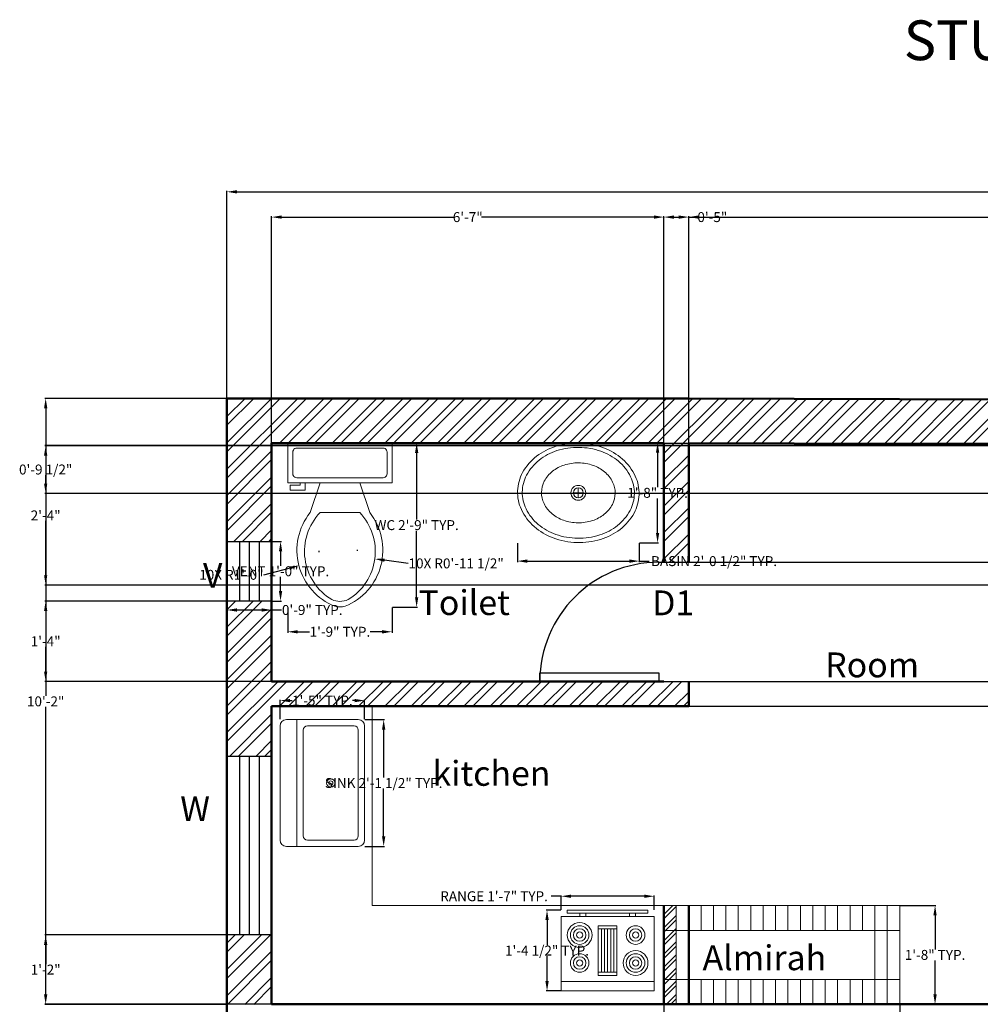
# Model space of a CAD drawing. Units: inches. Extents: x -83 to 408, y 158 to 919.
# Tile 3 of 5: x -83 to 111, y 721 to 919. Entities that reach past the tile are written whole.
import ezdxf

# ---------------------------------------------------------------- set-up
doc = ezdxf.new("R2010")
doc.units = ezdxf.units.IN
doc.header["$MEASUREMENT"] = 0
for name, color, linetype, lineweight in [('A-ANNO-DIMS', 2, 'Continuous', 18), ('A-ANNO-TEXT', 7, 'Continuous', 18), ('A-ANNO-TITL', 7, 'Continuous', 35), ('A-AREA-IDEN', 7, 'Continuous', 18), ('A-DOOR', 3, 'Continuous', 25), ('A-EQPM', 8, 'Continuous', 18), ('A-FLOR-CASE', 30, 'Continuous', 18), ('A-FLOR-FIXT', 9, 'Continuous', 18), ('A-GLAZ', 4, 'Continuous', 25), ('A-WALL', 7, 'Continuous', 50), ('A-WALL-PATT', 252, 'Continuous', 13)]:
    doc.layers.add(name, color=color, linetype=linetype, lineweight=lineweight)
doc.styles.get("Standard").update_dxf_attribs({"font": 'arial.ttf'})
doc.dimstyles.get("Standard").update_dxf_attribs({"dimtxt": 2, "dimasz": 2, "dimexe": 0.18, "dimexo": 0.0625, "dimgap": 0.09, "dimtad": 0, "dimtih": 1, "dimtoh": 1, "dimdec": 0, "dimzin": 0, "dimdsep": 46, "dimlunit": 3, "dimtxsty": 'Standard', "dimcen": 0.09, "dimadec": 0, "dimazin": 0, "dimtfac": 1, "dimtdec": 0, "dimtofl": 0, "dimtmove": 0, "dimatfit": 3, "dimfxl": 1, "dimtolj": 1, "dimtzin": 0, "dimarcsym": 0})

# ---------------------------------------------------------------- blocks, each defined once
blk = doc.blocks.new('Sink - Oval top')
for p, q in [((-1, 0), (1, 0)), ((0, 1), (0, -1))]:
    blk.add_line(p, q)
for points in [[(-12.23, 0.39, 0.117634), (-11.46, -3.36, 0.104469), (-8.88, -6.8, 0.090016), (-5.08, -9.07, 0.08192), (-0.32, -10.02, 0.08192), (4.49, -9.38, 0.090016), (8.42, -7.36, 0.104469), (11.22, -4.09, 0.117634), (12.23, -0.39, 0.117634), (11.46, 3.36, 0.104469), (8.88, 6.8, 0.090016), (5.08, 9.07, 0.08192), (0.32, 10.02, 0.08192), (-4.49, 9.38, 0.090016), (-8.42, 7.36, 0.104469), (-11.22, 4.09, 0.117634)], [(-11.29, 0.16, 0.118622), (-10.52, -3.25, 0.104678), (-8.07, -6.36, 0.089562), (-4.54, -8.37, 0.081185), (-0.13, -9.15, 0.081185), (4.3, -8.49, 0.089562), (7.89, -6.58, 0.104678), (10.42, -3.55, 0.118622), (11.29, -0.16, 0.118622), (10.52, 3.25, 0.104678), (8.07, 6.36, 0.089562), (4.54, 8.37, 0.081185), (0.13, 9.15, 0.081185), (-4.3, 8.49, 0.089562), (-7.89, 6.58, 0.104678), (-10.42, 3.55, 0.118622)], [(-7.42, 0.08, 0.118283), (-6.91, -2.17, 0.104607), (-5.29, -4.21, 0.089718), (-2.97, -5.53, 0.081436), (-0.07, -6.04, 0.081436), (2.84, -5.59, 0.089718), (5.2, -4.33, 0.104607), (6.86, -2.32, 0.118283), (7.42, -0.08, 0.118283), (6.91, 2.17, 0.104607), (5.29, 4.21, 0.089718), (2.97, 5.53, 0.081436), (0.07, 6.04, 0.081436), (-2.84, 5.59, 0.089718), (-5.2, 4.33, 0.104607), (-6.86, 2.32, 0.118283)]]:
    blk.add_lwpolyline(points, format="xyb", close=True)
for radius in [1.5, 1]:
    blk.add_circle((0, 0), radius)
blk = doc.blocks.new('Toilet - top')
for p, q in [((9.5, -6), (9.5, -2)), ((-10, -8.5), (-8, -8.5)), ((-10, -9.5), (-10, -8.5)), ((-7, -9.5), (-10, -9.5)), ((-8, -8.5), (-8, -8)), ((-7, -8), (-7, -9.5)), ((-4, -8), (-6, -14)), ((4, -8), (6, -14)), ((4, -14), (-4, -14))]:
    blk.add_line(p, q)
blk.add_lwpolyline([(10.5, -8), (10.5, 0), (-10.5, 0), (-10.5, -8)], close=True)
for points in [[(8.5, -1), (-8.5, -1)], [(-9.5, -2), (-9.5, -6)], [(-8.5, -7), (8.5, -7)]]:
    blk.add_lwpolyline(points)
for centre, radius, start, end in [((-8.62, -1.88), 0.884, 81.8699, 188.1301), ((8.62, -1.88), 0.884, 351.8699, 98.1301), ((-8.62, -6.12), 0.884, 171.8699, 278.1301), ((8.62, -6.12), 0.884, 261.8699, 8.1301), ((3.52, -21.58), 12.17, 141.4691, 247.9714), ((4.2, -21.82), 11.33, 136.3677, 238.9468), ((-3.52, -21.58), 12.17, 292.0284, 38.5307), ((-4.2, -21.82), 11.33, 301.053, 43.6321), ((0, -27.88), 4, 245.7318, 294.2682), ((0, -29), 4, 254.8605, 285.1395)]:
    blk.add_arc(centre, radius, start, end)
blk = doc.blocks.new('Sink-single - 30 in top')
blk.add_line((-15, -3.999996), (15, -3.999996))
for points in [[(-13.5, 0), (13.5, 0)], [(-15, -18.499996), (-15, -1.5)], [(15, -1.5), (15, -18.499996)], [(-13.5, -17.499996), (-13.5, -6.499996)], [(-12.5, -5.499996), (12.5, -5.499996)], [(13.5, -6.499996), (13.5, -17.499996)], [(12.5, -18.499996), (-12.5, -18.499996)], [(13.5, -19.999996), (-13.5, -19.999996)]]:
    blk.add_lwpolyline(points)
for radius in [1, 0.5]:
    blk.add_circle((0, -11.999996), radius)
for centre, radius, start, end in [((-13.5, -1.5), 1.5, 90, 180), ((13.5, -1.5), 1.5, 0, 90), ((-12.5, -6.499996), 1, 90, 180), ((12.5, -6.499996), 1, 0, 90), ((-13.5, -18.499996), 1.5, 180, 270), ((-12.5, -17.499996), 1, 180, 270), ((12.5, -17.499996), 1, 270, 0), ((13.5, -18.499996), 1.5, 270, 0)]:
    blk.add_arc(centre, radius, start, end)
blk = doc.blocks.new('Range-Oven - 30 in top')
for p, q in [((0, -3), (30, -3)), ((12, -6), (18, -6)), ((13, -20), (13, -6)), ((14, -6), (14, -20)), ((15, -20), (15, -6)), ((16, -6), (16, -20)), ((17, -20), (17, -6)), ((18, -20), (12, -20)), ((6, -24), (6, -25)), ((8, -25), (8, -24)), ((22, -25), (22, -24)), ((24, -24), (24, -25))]:
    blk.add_line(p, q)
for points in [[(0, -24), (0, 0), (30, 0), (30, -24)], [(12, -21), (12, -5), (18, -5), (18, -21)], [(2, -26), (2, -25), (28, -25), (28, -26)]]:
    blk.add_lwpolyline(points, close=True)
for centre, radius in [((6, -9), 4), ((6, -9), 3), ((24, -9), 3), ((6, -9), 2), ((6, -9), 1), ((24, -9), 2), ((24, -9), 1), ((6, -18), 3), ((24, -18), 4), ((24, -18), 3), ((6, -18), 2), ((6, -18), 1), ((24, -18), 2), ((24, -18), 1)]:
    blk.add_circle(centre, radius)
blk = doc.blocks.new('*U12')
for p, q in [((0, 0), (0, -6)), ((24, 0), (24, -6))]:
    blk.add_line(p, q)
blk.add_lwpolyline([(0, 0), (0, 24), (1.75, 24), (1.75, 0)], close=True)
blk.add_arc((0, 0), 24, 0, 90)
blk = doc.blocks.new('*D18')
at = {"layer": 'A-ANNO-DIMS', "color": 0, "lineweight": -2, "transparency": 16777216}
for p, q in [((-40.81, 843.26), (-40.81, 884.97)), ((-38.81, 884.79), (126.86, 884.79)), ((320.19, 884.79), (154.52, 884.79)), ((322.19, 842.73), (322.19, 884.97))]:
    blk.add_line(p, q, dxfattribs=at)
at = {"layer": 'A-ANNO-DIMS', "color": 0, "transparency": 16777216}
for points in [[(-38.81, 885.12), (-38.81, 884.46), (-40.81, 884.79)], [(320.19, 885.12), (320.19, 884.46), (322.19, 884.79)]]:
    blk.add_solid(points, dxfattribs=at)
at = {"layer": 'Defpoints', "color": 0, "transparency": 16777216}
for p in [(322.19, 884.79), (-40.81, 843.2), (322.19, 842.67)]:
    blk.add_point(p, dxfattribs=at)
at = {"layer": 'A-ANNO-DIMS', "color": 0, "transparency": 16777216, "insert": (140.69, 884.79), "char_height": 2, "attachment_point": 5}
blk.add_mtext('\\A1;{\\H4x;30\'-3"}', dxfattribs=at)
blk = doc.blocks.new('ALMIRAH-47IN')
for p, q in [((0, 19.88), (47.48, 19.88)), ((0, 19.88), (0, 0)), ((2.48, 19.88), (2.48, 0)), ((4.98, 19.88), (4.98, 0)), ((7.48, 19.88), (7.48, 14.88)), ((9.98, 19.88), (9.98, 14.88)), ((9.98, 19.88), (9.98, 14.88)), ((9.98, 19.88), (9.98, 14.88)), ((12.48, 19.88), (12.48, 14.88)), ((14.98, 19.88), (14.98, 14.88)), ((14.98, 19.88), (14.98, 14.88)), ((17.48, 19.88), (17.48, 14.88)), ((19.98, 19.88), (19.98, 14.88)), ((22.48, 19.88), (22.48, 14.88)), ((22.48, 19.88), (22.48, 14.88)), ((24.98, 19.88), (24.98, 14.88)), ((24.98, 19.88), (24.98, 14.88)), ((27.48, 19.88), (27.48, 14.88)), ((29.98, 19.88), (29.98, 14.88)), ((29.98, 19.88), (29.98, 14.88)), ((29.98, 19.88), (29.98, 14.88)), ((32.48, 19.88), (32.48, 14.88)), ((34.98, 19.88), (34.98, 14.88)), ((37.48, 19.88), (37.48, 14.88)), ((39.98, 19.88), (39.98, 14.88)), ((42.48, 19.88), (42.48, 0)), ((44.98, 19.88), (44.98, 0)), ((47.48, 19.88), (47.48, 0)), ((0, 14.88), (47.48, 14.88)), ((0, 5), (47.48, 5)), ((7.48, 5), (7.48, 0)), ((9.98, 5), (9.98, 0)), ((9.98, 5), (9.98, 0)), ((9.98, 5), (9.98, 0)), ((12.48, 5), (12.48, 0)), ((14.98, 5), (14.98, 0)), ((14.98, 5), (14.98, 0)), ((17.48, 5), (17.48, 0)), ((19.98, 5), (19.98, 0)), ((22.48, 5), (22.48, 0)), ((22.48, 5), (22.48, 0)), ((24.98, 5), (24.98, 0)), ((24.98, 5), (24.98, 0)), ((27.48, 5), (27.48, 0)), ((29.98, 5), (29.98, 0)), ((29.98, 5), (29.98, 0)), ((29.98, 5), (29.98, 0)), ((32.48, 5), (32.48, 0)), ((34.98, 5), (34.98, 0)), ((37.48, 5), (37.48, 0)), ((39.98, 5), (39.98, 0))]:
    blk.add_line(p, q)
blk = doc.blocks.new('WINDOW-36IN')
for p, q in [((2.5, 36), (2.5, 0)), ((4.5, 36), (4.5, 0)), ((6.5, 36), (6.5, 0))]:
    blk.add_line(p, q)
blk.add_lwpolyline([(0, 36), (9, 36), (9, 0), (0, 0)], close=True)
blk = doc.blocks.new('VENT-12IN')
for p, q in [((2.5, 12), (2.5, 0)), ((4.5, 12), (4.5, 0)), ((6.5, 12), (6.5, 0))]:
    blk.add_line(p, q)
blk.add_lwpolyline([(0, 12), (9, 12), (9, 0), (0, 0)], close=True)
blk = doc.blocks.new('COUNTER-L-STUDIO')
for p, q in [((0, 40.12), (0, 40.12)), ((0, 40.12), (0, 0)), ((0, 0), (63.78, 0))]:
    blk.add_line(p, q)
blk = doc.blocks.new('*D25')
at = {"layer": 'A-ANNO-DIMS', "color": 0, "lineweight": -2, "transparency": 16777216}
for p, q in [((-31.75, 814.39), (-29.83, 814.39)), ((-30.01, 812.39), (-30.01, 809.5)), ((-30.01, 804.39), (-30.01, 807.28)), ((-31.75, 802.39), (-29.83, 802.39))]:
    blk.add_line(p, q, dxfattribs=at)
at = {"layer": 'A-ANNO-DIMS', "color": 0, "transparency": 16777216}
for points in [[(-30.34, 812.39), (-29.68, 812.39), (-30.01, 814.39)], [(-30.34, 804.39), (-29.68, 804.39), (-30.01, 802.39)]]:
    blk.add_solid(points, dxfattribs=at)
at = {"layer": 'Defpoints', "color": 0, "transparency": 16777216}
for p in [(-31.81, 814.39), (-30.01, 814.39), (-31.81, 802.39)]:
    blk.add_point(p, dxfattribs=at)
at = {"layer": 'A-ANNO-DIMS', "color": 0, "transparency": 16777216, "insert": (-30.01, 808.39), "char_height": 2, "attachment_point": 5}
blk.add_mtext('\\A1;VENT 1\'-0" TYP.', dxfattribs=at)
blk = doc.blocks.new('*D26')
at = {"layer": 'A-ANNO-DIMS', "color": 0, "lineweight": -2, "transparency": 16777216}
for p, q in [((-40.81, 802.33), (-40.81, 800.41)), ((-31.81, 802.33), (-31.81, 800.41)), ((-38.81, 800.59), (-33.81, 800.59)), ((-31.81, 800.59), (-29.81, 800.59))]:
    blk.add_line(p, q, dxfattribs=at)
at = {"layer": 'A-ANNO-DIMS', "color": 0, "transparency": 16777216}
for points in [[(-38.81, 800.92), (-38.81, 800.25), (-40.81, 800.59)], [(-33.81, 800.92), (-33.81, 800.25), (-31.81, 800.59)]]:
    blk.add_solid(points, dxfattribs=at)
at = {"layer": 'Defpoints', "color": 0, "transparency": 16777216}
for p in [(-40.81, 802.39), (-31.81, 802.39), (-31.81, 800.59)]:
    blk.add_point(p, dxfattribs=at)
at = {"layer": 'A-ANNO-DIMS', "color": 0, "transparency": 16777216, "insert": (-23.63, 800.59), "char_height": 2, "attachment_point": 5}
blk.add_mtext('\\A1;0\'-9" TYP.', dxfattribs=at)
blk = doc.blocks.new('*D27')
at = {"layer": 'A-ANNO-DIMS', "color": 0, "lineweight": -2, "transparency": 16777216}
for p, q in [((17.68, 814.05), (17.68, 810.25)), ((42.23, 814.05), (42.23, 810.25)), ((19.68, 810.43), (40.23, 810.43)), ((42.23, 810.43), (44.23, 810.43))]:
    blk.add_line(p, q, dxfattribs=at)
at = {"layer": 'A-ANNO-DIMS', "color": 0, "transparency": 16777216}
for points in [[(19.68, 810.76), (19.68, 810.09), (17.68, 810.43)], [(40.23, 810.76), (40.23, 810.09), (42.23, 810.43)]]:
    blk.add_solid(points, dxfattribs=at)
at = {"layer": 'Defpoints', "color": 0, "transparency": 16777216}
for p in [(17.68, 814.11), (42.23, 814.11), (42.23, 810.43)]:
    blk.add_point(p, dxfattribs=at)
at = {"layer": 'A-ANNO-DIMS', "color": 0, "transparency": 16777216, "insert": (57.28, 810.43), "char_height": 2, "attachment_point": 5}
blk.add_mtext('\\A1;BASIN 2\'-0 1/2" TYP.', dxfattribs=at)
blk = doc.blocks.new('*D28')
at = {"layer": 'A-ANNO-DIMS', "color": 0, "lineweight": -2, "transparency": 16777216}
for p, q in [((42.29, 834.25), (46.09, 834.25)), ((45.91, 832.25), (45.91, 825.29)), ((45.91, 816.11), (45.91, 823.07)), ((42.29, 814.11), (46.09, 814.11))]:
    blk.add_line(p, q, dxfattribs=at)
at = {"layer": 'A-ANNO-DIMS', "color": 0, "transparency": 16777216}
for points in [[(45.58, 832.25), (46.24, 832.25), (45.91, 834.25)], [(45.58, 816.11), (46.24, 816.11), (45.91, 814.11)]]:
    blk.add_solid(points, dxfattribs=at)
at = {"layer": 'Defpoints', "color": 0, "transparency": 16777216}
for p in [(42.23, 834.25), (45.91, 834.25), (42.23, 814.11)]:
    blk.add_point(p, dxfattribs=at)
at = {"layer": 'A-ANNO-DIMS', "color": 0, "transparency": 16777216, "insert": (45.91, 824.18), "char_height": 2, "attachment_point": 5}
blk.add_mtext('\\A1;1\'-8" TYP.', dxfattribs=at)
blk = doc.blocks.new('*D29')
at = {"layer": 'A-ANNO-DIMS', "color": 0, "lineweight": -2, "transparency": 16777216}
for p, q in [((-7.5, 834.2), (-2.43, 834.2)), ((-2.61, 832.2), (-2.61, 818.8)), ((-2.61, 803.15), (-2.61, 816.55)), ((-7.5, 801.15), (-2.43, 801.15))]:
    blk.add_line(p, q, dxfattribs=at)
at = {"layer": 'A-ANNO-DIMS', "color": 0, "transparency": 16777216}
for points in [[(-2.94, 832.2), (-2.27, 832.2), (-2.61, 834.2)], [(-2.94, 803.15), (-2.27, 803.15), (-2.61, 801.15)]]:
    blk.add_solid(points, dxfattribs=at)
at = {"layer": 'Defpoints', "color": 0, "transparency": 16777216}
for p in [(-7.56, 834.2), (-2.61, 834.2), (-7.56, 801.15)]:
    blk.add_point(p, dxfattribs=at)
at = {"layer": 'A-ANNO-DIMS', "color": 0, "transparency": 16777216, "insert": (-2.61, 817.68), "char_height": 2, "attachment_point": 5}
blk.add_mtext('\\A1;WC 2\'-9" TYP.', dxfattribs=at)
blk = doc.blocks.new('*D30')
at = {"layer": 'A-ANNO-DIMS', "color": 0, "lineweight": -2, "transparency": 16777216}
for p, q in [((-28.56, 801.09), (-28.56, 796.02)), ((-7.56, 801.09), (-7.56, 796.02)), ((-26.56, 796.2), (-24.15, 796.2)), ((-9.56, 796.2), (-11.97, 796.2))]:
    blk.add_line(p, q, dxfattribs=at)
at = {"layer": 'A-ANNO-DIMS', "color": 0, "transparency": 16777216}
for points in [[(-26.56, 796.53), (-26.56, 795.86), (-28.56, 796.2)], [(-9.56, 796.53), (-9.56, 795.86), (-7.56, 796.2)]]:
    blk.add_solid(points, dxfattribs=at)
at = {"layer": 'Defpoints', "color": 0, "transparency": 16777216}
for p in [(-28.56, 801.15), (-7.56, 801.15), (-7.56, 796.2)]:
    blk.add_point(p, dxfattribs=at)
at = {"layer": 'A-ANNO-DIMS', "color": 0, "transparency": 16777216, "insert": (-18.06, 796.2), "char_height": 2, "attachment_point": 5}
blk.add_mtext('\\A1;1\'-9" TYP.', dxfattribs=at)
blk = doc.blocks.new('*D33')
at = {"layer": 'A-ANNO-DIMS', "color": 0, "lineweight": -2, "transparency": 16777216}
for p, q in [((-13.02, 778.52), (-9.07, 778.52)), ((-9.25, 776.52), (-9.25, 766.87)), ((-9.25, 754.98), (-9.25, 764.62)), ((-13.02, 752.98), (-9.07, 752.98))]:
    blk.add_line(p, q, dxfattribs=at)
at = {"layer": 'A-ANNO-DIMS', "color": 0, "transparency": 16777216}
for points in [[(-9.58, 776.52), (-8.92, 776.52), (-9.25, 778.52)], [(-9.58, 754.98), (-8.92, 754.98), (-9.25, 752.98)]]:
    blk.add_solid(points, dxfattribs=at)
at = {"layer": 'Defpoints', "color": 0, "transparency": 16777216}
for p in [(-13.08, 778.52), (-9.25, 778.52), (-13.08, 752.98)]:
    blk.add_point(p, dxfattribs=at)
at = {"layer": 'A-ANNO-DIMS', "color": 0, "transparency": 16777216, "insert": (-9.25, 765.75), "char_height": 2, "attachment_point": 5}
blk.add_mtext('\\A1;SINK 2\'-1 1/2" TYP.', dxfattribs=at)
blk = doc.blocks.new('*D34')
at = {"layer": 'A-ANNO-DIMS', "color": 0, "lineweight": -2, "transparency": 16777216}
for p, q in [((-30.11, 778.58), (-30.11, 782.53)), ((-28.11, 782.35), (-27.69, 782.35)), ((-15.08, 782.35), (-15.5, 782.35)), ((-13.08, 778.58), (-13.08, 782.53))]:
    blk.add_line(p, q, dxfattribs=at)
at = {"layer": 'A-ANNO-DIMS', "color": 0, "transparency": 16777216}
for points in [[(-28.11, 782.68), (-28.11, 782.02), (-30.11, 782.35)], [(-15.08, 782.68), (-15.08, 782.02), (-13.08, 782.35)]]:
    blk.add_solid(points, dxfattribs=at)
at = {"layer": 'Defpoints', "color": 0, "transparency": 16777216}
for p in [(-30.11, 782.35), (-30.11, 778.52), (-13.08, 778.52)]:
    blk.add_point(p, dxfattribs=at)
at = {"layer": 'A-ANNO-DIMS', "color": 0, "transparency": 16777216, "insert": (-21.6, 782.35), "char_height": 2, "attachment_point": 5}
blk.add_mtext('\\A1;1\'-5" TYP.', dxfattribs=at)
blk = doc.blocks.new('*D35')
at = {"layer": 'A-ANNO-DIMS', "color": 0, "lineweight": -2, "transparency": 16777216}
for p, q in [((26.47, 742.95), (24.47, 742.95)), ((26.47, 740.2), (26.47, 743.13)), ((43.23, 742.95), (28.47, 742.95)), ((45.23, 740.2), (45.23, 743.13))]:
    blk.add_line(p, q, dxfattribs=at)
at = {"layer": 'A-ANNO-DIMS', "color": 0, "transparency": 16777216}
for points in [[(28.47, 743.28), (28.47, 742.62), (26.47, 742.95)], [(43.23, 743.28), (43.23, 742.62), (45.23, 742.95)]]:
    blk.add_solid(points, dxfattribs=at)
at = {"layer": 'Defpoints', "color": 0, "transparency": 16777216}
for p in [(26.47, 742.95), (26.47, 740.14), (45.23, 740.14)]:
    blk.add_point(p, dxfattribs=at)
at = {"layer": 'A-ANNO-DIMS', "color": 0, "transparency": 16777216, "insert": (12.98, 742.95), "char_height": 2, "attachment_point": 5}
blk.add_mtext('\\A1;RANGE 1\'-7" TYP.', dxfattribs=at)
blk = doc.blocks.new('*D36')
at = {"layer": 'A-ANNO-DIMS', "color": 0, "lineweight": -2, "transparency": 16777216}
for p, q in [((26.4, 740.14), (23.47, 740.14)), ((23.65, 738.14), (23.65, 733.13)), ((23.65, 725.88), (23.65, 730.88)), ((26.4, 723.88), (23.47, 723.88))]:
    blk.add_line(p, q, dxfattribs=at)
at = {"layer": 'A-ANNO-DIMS', "color": 0, "transparency": 16777216}
for points in [[(23.32, 738.14), (23.99, 738.14), (23.65, 740.14)], [(23.32, 725.88), (23.99, 725.88), (23.65, 723.88)]]:
    blk.add_solid(points, dxfattribs=at)
at = {"layer": 'Defpoints', "color": 0, "transparency": 16777216}
for p in [(26.47, 740.14), (23.65, 723.88), (26.47, 723.88)]:
    blk.add_point(p, dxfattribs=at)
at = {"layer": 'A-ANNO-DIMS', "color": 0, "transparency": 16777216, "insert": (23.65, 732.01), "char_height": 2, "attachment_point": 5}
blk.add_mtext('\\A1;1\'-4 1/2" TYP.', dxfattribs=at)
blk = doc.blocks.new('*D37')
at = {"layer": 'A-ANNO-DIMS', "color": 0, "lineweight": -2, "transparency": 16777216}
for p, q in [((47.19, 721.14), (47.19, 713.9)), ((94.67, 721.14), (94.67, 713.9)), ((49.19, 714.08), (52.98, 714.08)), ((92.67, 714.08), (88.88, 714.08))]:
    blk.add_line(p, q, dxfattribs=at)
at = {"layer": 'A-ANNO-DIMS', "color": 0, "transparency": 16777216}
for points in [[(49.19, 714.41), (49.19, 713.75), (47.19, 714.08)], [(92.67, 714.41), (92.67, 713.75), (94.67, 714.08)]]:
    blk.add_solid(points, dxfattribs=at)
at = {"layer": 'Defpoints', "color": 0, "transparency": 16777216}
for p in [(47.19, 721.2), (94.67, 721.2), (94.67, 714.08)]:
    blk.add_point(p, dxfattribs=at)
at = {"layer": 'A-ANNO-DIMS', "color": 0, "transparency": 16777216, "insert": (70.93, 714.08), "char_height": 2, "attachment_point": 5}
blk.add_mtext('\\A1;WARDROBE 3\'-11 1/2" TYP.', dxfattribs=at)
blk = doc.blocks.new('*D38')
at = {"layer": 'A-ANNO-DIMS', "color": 0, "lineweight": -2, "transparency": 16777216}
for p, q in [((94.73, 741.08), (101.97, 741.08)), ((101.79, 739.08), (101.79, 732.25)), ((101.79, 723.2), (101.79, 730.03)), ((94.73, 721.2), (101.97, 721.2))]:
    blk.add_line(p, q, dxfattribs=at)
at = {"layer": 'A-ANNO-DIMS', "color": 0, "transparency": 16777216}
for points in [[(101.45, 739.08), (102.12, 739.08), (101.79, 741.08)], [(101.45, 723.2), (102.12, 723.2), (101.79, 721.2)]]:
    blk.add_solid(points, dxfattribs=at)
at = {"layer": 'Defpoints', "color": 0, "transparency": 16777216}
for p in [(94.67, 741.08), (101.79, 741.08), (94.67, 721.2)]:
    blk.add_point(p, dxfattribs=at)
at = {"layer": 'A-ANNO-DIMS', "color": 0, "transparency": 16777216, "insert": (101.79, 731.14), "char_height": 2, "attachment_point": 5}
blk.add_mtext('\\A1;1\'-8" TYP.', dxfattribs=at)
blk = doc.blocks.new('*D42')
at = {"layer": 'A-ANNO-DIMS', "color": 0, "lineweight": -2, "transparency": 16777216}
for p, q in [((-40.87, 843.2), (-77.49, 843.2)), ((-77.31, 841.2), (-77.31, 783.3)), ((-77.31, 723.18), (-77.31, 781.08)), ((-40.87, 721.18), (-77.49, 721.18))]:
    blk.add_line(p, q, dxfattribs=at)
at = {"layer": 'A-ANNO-DIMS', "color": 0, "transparency": 16777216}
for points in [[(-77.64, 841.2), (-76.98, 841.2), (-77.31, 843.2)], [(-77.64, 723.18), (-76.98, 723.18), (-77.31, 721.18)]]:
    blk.add_solid(points, dxfattribs=at)
at = {"layer": 'Defpoints', "color": 0, "transparency": 16777216}
for p in [(-40.81, 843.2), (-77.31, 721.18), (-40.81, 721.18)]:
    blk.add_point(p, dxfattribs=at)
at = {"layer": 'A-ANNO-DIMS', "color": 0, "transparency": 16777216, "insert": (-77.31, 782.19), "char_height": 2, "attachment_point": 5}
blk.add_mtext('\\A1;10\'-2"', dxfattribs=at)
blk = doc.blocks.new('*D47')
at = {"layer": 'A-ANNO-DIMS', "color": 0, "lineweight": -2, "transparency": 16777216}
for p, q in [((-31.81, 834.26), (-31.81, 879.88)), ((-29.81, 879.7), (4.94, 879.7)), ((45.19, 879.7), (10.44, 879.7)), ((47.19, 834.26), (47.19, 879.88))]:
    blk.add_line(p, q, dxfattribs=at)
at = {"layer": 'A-ANNO-DIMS', "color": 0, "transparency": 16777216}
for points in [[(-29.81, 880.03), (-29.81, 879.37), (-31.81, 879.7)], [(45.19, 880.03), (45.19, 879.37), (47.19, 879.7)]]:
    blk.add_solid(points, dxfattribs=at)
at = {"layer": 'Defpoints', "color": 0, "transparency": 16777216}
for p in [(47.19, 879.7), (-31.81, 834.2), (47.19, 834.2)]:
    blk.add_point(p, dxfattribs=at)
at = {"layer": 'A-ANNO-DIMS', "color": 0, "transparency": 16777216, "insert": (7.69, 879.7), "char_height": 2, "attachment_point": 5}
blk.add_mtext('\\A1;6\'-7"', dxfattribs=at)
blk = doc.blocks.new('*D48')
at = {"layer": 'A-ANNO-DIMS', "color": 0, "lineweight": -2, "transparency": 16777216}
for p, q in [((47.25, 834.2), (358.87, 834.2)), ((358.69, 832.2), (358.69, 811.31)), ((358.69, 788.2), (358.69, 809.09)), ((47.25, 786.2), (358.87, 786.2))]:
    blk.add_line(p, q, dxfattribs=at)
at = {"layer": 'A-ANNO-DIMS', "color": 0, "transparency": 16777216}
for points in [[(358.36, 832.2), (359.02, 832.2), (358.69, 834.2)], [(358.36, 788.2), (359.02, 788.2), (358.69, 786.2)]]:
    blk.add_solid(points, dxfattribs=at)
at = {"layer": 'Defpoints', "color": 0, "transparency": 16777216}
for p in [(47.19, 834.2), (47.19, 786.2), (358.69, 786.2)]:
    blk.add_point(p, dxfattribs=at)
at = {"layer": 'A-ANNO-DIMS', "color": 0, "transparency": 16777216, "insert": (358.69, 810.2), "char_height": 2, "attachment_point": 5}
blk.add_mtext('\\A1;4\'-0"', dxfattribs=at)
blk = doc.blocks.new('*D49')
at = {"layer": 'A-ANNO-DIMS', "color": 0, "lineweight": -2, "transparency": 16777216}
for p, q in [((47.25, 810.2), (358.87, 810.2)), ((358.69, 808.2), (358.69, 799.31)), ((358.69, 788.2), (358.69, 797.09)), ((47.25, 786.2), (358.87, 786.2))]:
    blk.add_line(p, q, dxfattribs=at)
at = {"layer": 'A-ANNO-DIMS', "color": 0, "transparency": 16777216}
for points in [[(358.36, 808.2), (359.02, 808.2), (358.69, 810.2)], [(358.36, 788.2), (359.02, 788.2), (358.69, 786.2)]]:
    blk.add_solid(points, dxfattribs=at)
at = {"layer": 'Defpoints', "color": 0, "transparency": 16777216}
for p in [(47.19, 810.2), (47.19, 786.2), (358.69, 786.2)]:
    blk.add_point(p, dxfattribs=at)
at = {"layer": 'A-ANNO-DIMS', "color": 0, "transparency": 16777216, "insert": (358.69, 798.2), "char_height": 2, "attachment_point": 5}
blk.add_mtext('\\A1;2\'-0"', dxfattribs=at)
blk = doc.blocks.new('*D51')
at = {"layer": 'A-ANNO-DIMS', "color": 0, "lineweight": -2, "transparency": 16777216}
for p, q in [((52.19, 834.26), (52.19, 879.88)), ((54.19, 879.7), (119.26, 879.7)), ((191.19, 879.7), (126.12, 879.7)), ((193.19, 833.76), (193.19, 879.88))]:
    blk.add_line(p, q, dxfattribs=at)
at = {"layer": 'A-ANNO-DIMS', "color": 0, "transparency": 16777216}
for points in [[(54.19, 880.03), (54.19, 879.37), (52.19, 879.7)], [(191.19, 880.03), (191.19, 879.37), (193.19, 879.7)]]:
    blk.add_solid(points, dxfattribs=at)
at = {"layer": 'Defpoints', "color": 0, "transparency": 16777216}
for p in [(193.19, 879.7), (52.19, 834.2), (193.19, 833.7)]:
    blk.add_point(p, dxfattribs=at)
at = {"layer": 'A-ANNO-DIMS', "color": 0, "transparency": 16777216, "insert": (122.69, 879.7), "char_height": 2, "attachment_point": 5}
blk.add_mtext('\\A1;11\'-9"', dxfattribs=at)
blk = doc.blocks.new('*D52')
at = {"layer": 'A-ANNO-DIMS', "color": 0, "lineweight": -2, "transparency": 16777216}
for p, q in [((-31.87, 735.16), (-77.49, 735.16)), ((-77.31, 733.16), (-77.31, 729.27)), ((-77.31, 723.2), (-77.31, 727.09)), ((-31.87, 721.2), (-77.49, 721.2))]:
    blk.add_line(p, q, dxfattribs=at)
at = {"layer": 'A-ANNO-DIMS', "color": 0, "transparency": 16777216}
for points in [[(-77.64, 733.16), (-76.98, 733.16), (-77.31, 735.16)], [(-77.64, 723.2), (-76.98, 723.2), (-77.31, 721.2)]]:
    blk.add_solid(points, dxfattribs=at)
at = {"layer": 'Defpoints', "color": 0, "transparency": 16777216}
for p in [(-31.81, 735.16), (-77.31, 721.2), (-31.81, 721.2)]:
    blk.add_point(p, dxfattribs=at)
at = {"layer": 'A-ANNO-DIMS', "color": 0, "transparency": 16777216, "insert": (-77.31, 728.18), "char_height": 2, "attachment_point": 5}
blk.add_mtext('\\A1;1\'-2"', dxfattribs=at)
blk = doc.blocks.new('*D53')
at = {"layer": 'A-ANNO-DIMS', "color": 0, "lineweight": -2, "transparency": 16777216}
for p, q in [((-31.87, 802.39), (-77.49, 802.39)), ((-77.31, 800.39), (-77.31, 795.39)), ((-77.31, 788.2), (-77.31, 793.2)), ((-31.87, 786.2), (-77.49, 786.2))]:
    blk.add_line(p, q, dxfattribs=at)
at = {"layer": 'A-ANNO-DIMS', "color": 0, "transparency": 16777216}
for points in [[(-77.64, 800.39), (-76.98, 800.39), (-77.31, 802.39)], [(-77.64, 788.2), (-76.98, 788.2), (-77.31, 786.2)]]:
    blk.add_solid(points, dxfattribs=at)
at = {"layer": 'Defpoints', "color": 0, "transparency": 16777216}
for p in [(-31.81, 802.39), (-77.31, 786.2), (-31.81, 786.2)]:
    blk.add_point(p, dxfattribs=at)
at = {"layer": 'A-ANNO-DIMS', "color": 0, "transparency": 16777216, "insert": (-77.31, 794.29), "char_height": 2, "attachment_point": 5}
blk.add_mtext('\\A1;1\'-4"', dxfattribs=at)
blk = doc.blocks.new('*D55')
at = {"layer": 'A-ANNO-DIMS', "color": 0, "lineweight": -2, "transparency": 16777216}
for p, q in [((47.19, 834.26), (47.19, 879.88)), ((49.19, 879.7), (50.19, 879.7)), ((52.19, 834.26), (52.19, 879.88)), ((52.19, 879.7), (54.19, 879.7))]:
    blk.add_line(p, q, dxfattribs=at)
at = {"layer": 'A-ANNO-DIMS', "color": 0, "transparency": 16777216}
for points in [[(49.19, 880.03), (49.19, 879.37), (47.19, 879.7)], [(50.19, 880.03), (50.19, 879.37), (52.19, 879.7)]]:
    blk.add_solid(points, dxfattribs=at)
at = {"layer": 'Defpoints', "color": 0, "transparency": 16777216}
for p in [(52.19, 879.7), (47.19, 834.2), (52.19, 834.2)]:
    blk.add_point(p, dxfattribs=at)
at = {"layer": 'A-ANNO-DIMS', "color": 0, "transparency": 16777216, "insert": (56.94, 879.7), "char_height": 2, "attachment_point": 5}
blk.add_mtext('\\A1;0\'-5"', dxfattribs=at)
blk = doc.blocks.new('*D56')
at = {"layer": 'A-ANNO-DIMS', "color": 0, "lineweight": -2, "transparency": 16777216}
for p, q in [((52.25, 781.2), (358.87, 781.2)), ((358.69, 779.2), (358.69, 752.31)), ((358.69, 723.2), (358.69, 750.09)), ((47.25, 721.2), (358.87, 721.2))]:
    blk.add_line(p, q, dxfattribs=at)
at = {"layer": 'A-ANNO-DIMS', "color": 0, "transparency": 16777216}
for points in [[(358.36, 779.2), (359.02, 779.2), (358.69, 781.2)], [(358.36, 723.2), (359.02, 723.2), (358.69, 721.2)]]:
    blk.add_solid(points, dxfattribs=at)
at = {"layer": 'Defpoints', "color": 0, "transparency": 16777216}
for p in [(52.19, 781.2), (47.19, 721.2), (358.69, 721.2)]:
    blk.add_point(p, dxfattribs=at)
at = {"layer": 'A-ANNO-DIMS', "color": 0, "transparency": 16777216, "insert": (358.69, 751.2), "char_height": 2, "attachment_point": 5}
blk.add_mtext('\\A1;5\'-0"', dxfattribs=at)
blk = doc.blocks.new('*D62')
at = {"layer": 'A-ANNO-DIMS', "color": 0, "lineweight": -2, "transparency": 16777216}
for p, q in [((272.31, 833.67), (-77.49, 833.67)), ((-77.31, 831.67), (-77.31, 820.72)), ((-77.31, 807.59), (-77.31, 818.54)), ((274.13, 805.59), (-77.49, 805.59))]:
    blk.add_line(p, q, dxfattribs=at)
at = {"layer": 'A-ANNO-DIMS', "color": 0, "transparency": 16777216}
for points in [[(-77.64, 831.67), (-76.98, 831.67), (-77.31, 833.67)], [(-77.64, 807.59), (-76.98, 807.59), (-77.31, 805.59)]]:
    blk.add_solid(points, dxfattribs=at)
at = {"layer": 'Defpoints', "color": 0, "transparency": 16777216}
for p in [(-77.31, 833.67), (272.37, 833.67), (274.19, 805.59)]:
    blk.add_point(p, dxfattribs=at)
at = {"layer": 'A-ANNO-DIMS', "color": 0, "transparency": 16777216, "insert": (-77.31, 819.63), "char_height": 2, "attachment_point": 5}
blk.add_mtext('\\A1;2\'-4"', dxfattribs=at)
blk = doc.blocks.new('*D72')
at = {"layer": 'A-ANNO-DIMS', "color": 0, "lineweight": -2, "transparency": 16777216}
for p, q in [((193.13, 833.7), (-77.49, 833.7)), ((-77.31, 831.7), (-77.31, 829.99)), ((-77.31, 826.04), (-77.31, 827.74)), ((128.21, 824.04), (-77.49, 824.04))]:
    blk.add_line(p, q, dxfattribs=at)
at = {"layer": 'A-ANNO-DIMS', "color": 0, "transparency": 16777216}
for points in [[(-77.64, 831.7), (-76.98, 831.7), (-77.31, 833.7)], [(-77.64, 826.04), (-76.98, 826.04), (-77.31, 824.04)]]:
    blk.add_solid(points, dxfattribs=at)
at = {"layer": 'Defpoints', "color": 0, "transparency": 16777216}
for p in [(-77.31, 833.7), (193.19, 833.7), (128.28, 824.04)]:
    blk.add_point(p, dxfattribs=at)
at = {"layer": 'A-ANNO-DIMS', "color": 0, "transparency": 16777216, "insert": (-77.31, 828.87), "char_height": 2, "attachment_point": 5}
blk.add_mtext('\\A1;0\'-9 1/2"', dxfattribs=at)
blk = doc.blocks.new('*D73')
at = {"layer": 'A-ANNO-DIMS', "color": 0, "lineweight": -2, "transparency": 16777216}
for p, q in [((-14.63, 812.62), (-14.45, 812.62)), ((-14.54, 812.53), (-14.54, 812.71)), ((-33.37, 807.67), (-28.25, 809.02))]:
    blk.add_line(p, q, dxfattribs=at)
at = {"layer": 'A-ANNO-DIMS', "color": 0, "transparency": 16777216}
blk.add_solid([(-28.33, 809.34), (-28.16, 808.7), (-26.31, 809.53)], dxfattribs=at)
at = {"layer": 'Defpoints', "color": 0, "transparency": 16777216}
for p in [(-14.54, 812.62), (-26.31, 809.53)]:
    blk.add_point(p, dxfattribs=at)
at = {"layer": 'A-ANNO-DIMS', "color": 0, "transparency": 16777216, "insert": (-39.91, 807.67), "char_height": 2, "attachment_point": 5}
blk.add_mtext('\\A1;10X R1\'-0"', dxfattribs=at)
blk = doc.blocks.new('*D74')
at = {"layer": 'A-ANNO-DIMS', "color": 0, "lineweight": -2, "transparency": 16777216}
for p, q in [((-22.35, 812.38), (-22.17, 812.38)), ((-22.26, 812.29), (-22.26, 812.47)), ((-4.3, 809.97), (-9.05, 810.61))]:
    blk.add_line(p, q, dxfattribs=at)
at = {"layer": 'A-ANNO-DIMS', "color": 0, "transparency": 16777216}
blk.add_solid([(-9.01, 810.94), (-9.1, 810.28), (-11.03, 810.87)], dxfattribs=at)
at = {"layer": 'Defpoints', "color": 0, "transparency": 16777216}
for p in [(-22.26, 812.38), (-11.03, 810.87)]:
    blk.add_point(p, dxfattribs=at)
at = {"layer": 'A-ANNO-DIMS', "color": 0, "transparency": 16777216, "insert": (5.35, 809.97), "char_height": 2, "attachment_point": 5}
blk.add_mtext('\\A1;10X R0\'-11 1/2"', dxfattribs=at)

msp = doc.modelspace()

# ---------------------------------------------------------------- hatches: boundary and pattern name
at = {"layer": 'A-WALL-PATT'}
h = msp.add_hatch(dxfattribs=at)
h.set_pattern_fill('ANSI32', color=256, scale=10)
h.paths.add_polyline_path([(202.19, 842.67), (52.21, 843.2), (-40.81, 843.2), (-40.81, 814.39), (-31.81, 814.39), (-31.81, 834.2), (47.19, 834.2), (47.19, 810.2), (52.19, 810.2), (52.19, 834.2), (193.19, 833.7), (193.19, 811.95), (202.19, 811.95)])
h.paths.add_polyline_path([(-31.81, 781.2), (52.19, 781.2), (52.19, 786.2), (46.19, 786.2), (22.19, 786.2), (-31.81, 786.2), (-31.81, 802.39), (-40.81, 802.39), (-40.81, 771.16), (-31.81, 771.16)])
h.paths.add_polyline_path([(-31.81, 735.16), (-40.81, 735.16), (-40.81, 721.18), (-31.81, 721.18)])
h.paths.add_polyline_path([(202.19, 775.95), (193.19, 775.95), (193.19, 757.08, -0.020861), (196.19, 757.2), (202.19, 757.2)])
h = msp.add_hatch(dxfattribs=at)
h.set_pattern_fill('ANSI32', color=256, scale=5)
h.paths.add_polyline_path([(49.67, 736.08), (47.19, 736.08), (47.19, 726.2), (49.67, 726.2)])
h.paths.add_polyline_path([(49.67, 726.2), (47.19, 726.2), (47.19, 721.2), (49.67, 721.2)])
h.paths.add_polyline_path([(49.67, 741.08), (47.19, 741.08), (47.19, 736.08), (49.67, 736.08)])

# ---------------------------------------------------------------- linework, layer by layer
at = {"layer": 'A-WALL'}
for p, q in [((-40.81, 712.2), (-40.81, 843.2)), ((-40.81, 843.2), (52.19, 843.2)), ((202.19, 842.67), (52.22, 843.2)), ((-31.81, 834.2), (47.19, 834.2)), ((-31.81, 786.2), (-31.81, 834.2)), ((47.19, 834.2), (47.19, 810.2)), ((52.19, 834.2), (52.19, 810.2)), ((193.19, 833.7), (52.19, 834.2)), ((52.19, 834.2), (52.19, 810.2)), ((47.19, 786.2), (-31.81, 786.2)), ((-31.81, 786.2), (47.19, 786.2)), ((52.19, 786.2), (52.19, 781.2)), ((52.19, 786.2), (52.19, 781.2)), ((47.19, 781.2), (-31.81, 781.2)), ((-31.81, 781.2), (52.19, 781.2)), ((-31.81, 721.2), (-31.81, 781.2)), ((47.19, 741.08), (47.19, 721.2)), ((52.19, 741.08), (52.19, 721.2)), ((47.19, 721.2), (-31.81, 721.2)), ((47.19, 721.2), (193.19, 721.2))]:
    msp.add_line(p, q, dxfattribs=at)

# ---------------------------------------------------------------- block references
at = {"layer": 'A-DOOR', "rotation": 90}
msp.add_blockref('*U12', (46.19, 786.2), dxfattribs=at)
at = {"layer": 'A-EQPM', "xscale": 0.6253442555691314, "yscale": 0.6253442555691314, "zscale": 0.6253442555691314, "rotation": 180}
msp.add_blockref('Range-Oven - 30 in top', (45.23, 723.88), dxfattribs=at)
at = {"layer": 'A-FLOR-CASE'}
for name, p in [('COUNTER-L-STUDIO', (-11.59, 741.09)), ('ALMIRAH-47IN', (47.19, 721.2))]:
    msp.add_blockref(name, p, dxfattribs=at)
at = {"layer": 'A-FLOR-FIXT'}
for name, p in [('Toilet - top', (-18.06, 834.2)), ('Sink - Oval top', (29.95, 824.18))]:
    msp.add_blockref(name, p, dxfattribs=at)
at = {"layer": 'A-FLOR-FIXT', "xscale": 0.8513407291768876, "yscale": 0.8513407291768876, "zscale": 0.8513407291768876, "rotation": 90}
msp.add_blockref('Sink-single - 30 in top', (-30.11, 765.75), dxfattribs=at)
at = {"layer": 'A-GLAZ'}
for name, p in [('VENT-12IN', (-40.81, 802.39)), ('WINDOW-36IN', (-40.81, 735.16))]:
    msp.add_blockref(name, p, dxfattribs=at)

# ---------------------------------------------------------------- texts
at = {"layer": 'A-ANNO-TEXT', "char_height": 5, "attachment_point": 1}
for s, width, insert in [('V', 4.2263, (-45.64, 810.07)), ('D1', 13.3697, (44.82, 804.52)), ('W', 4.9358, (-50.22, 763.08)), ('Almirah', 24.1185, (54.97, 733.06))]:
    msp.add_mtext_dynamic_manual_height_columns(s, width=width, gutter_width=1, heights=[0], dxfattribs=dict(at, insert=insert))
at = {"layer": 'A-ANNO-TITL', "insert": (95.49, 919.3), "char_height": 8, "attachment_point": 1}
msp.add_mtext_dynamic_manual_height_columns('STUDIO UNIT  APARTMENT', width=288.4341, gutter_width=1, heights=[0], dxfattribs=at)
at = {"layer": 'A-AREA-IDEN', "char_height": 5, "attachment_point": 1}
for s, width, heights, insert in [('Toilet', 21.3997, [0.203], (-2.22, 804.57)), ('Room', 29.7735, [0], (79.66, 792.03)), ('kitchen', 18.1432, [0], (0.57, 770.19))]:
    msp.add_mtext_dynamic_manual_height_columns(s, width=width, gutter_width=1, heights=heights, dxfattribs=dict(at, insert=insert))

# ---------------------------------------------------------------- dimensions: what is measured, and where the dimension line sits
at = {"layer": 'A-ANNO-DIMS'}
for base, p1, p2, text, override, picture, middle in [((322.19, 884.79), (-40.81, 843.2), (322.19, 842.67), '{\\H4x;<>}', {"dimclrd": 0, "dimclre": 0, "dimclrt": 0}, '*D18', (140.69, 884.79)), ((42.2281, 810.4258), (17.6772, 814.1084), (42.2281, 814.1084), 'BASIN <> TYP.', {"dimdec": 1, "dimlfac": 1, "dimrnd": 0, "dimzin": 1, "dimdsep": 46, "dimlunit": 4, "dimfrac": 2}, '*D27', (57.2799, 810.4258)), ((-31.81, 800.59), (-40.81, 802.39), (-31.81, 802.39), '<> TYP.', {"dimdec": 1, "dimlfac": 1, "dimrnd": 0, "dimzin": 1, "dimdsep": 46, "dimlunit": 4, "dimfrac": 2}, '*D26', (-23.63, 800.59)), ((-7.56, 796.2), (-28.56, 801.15), (-7.56, 801.15), '<> TYP.', {"dimdec": 1, "dimlfac": 1, "dimrnd": 0, "dimzin": 1, "dimdsep": 46, "dimlunit": 4, "dimfrac": 2}, '*D30', (-18.06, 796.2)), ((94.67, 714.08), (47.19, 721.2), (94.67, 721.2), 'WARDROBE <> TYP.', {"dimdec": 1, "dimlfac": 1, "dimrnd": 0, "dimzin": 1, "dimdsep": 46, "dimlunit": 4, "dimfrac": 2}, '*D37', (70.93, 714.08))]:
    dim = msp.add_linear_dim(base=base, p1=p1, p2=p2, text=text, dimstyle='Standard', override=override, dxfattribs=at)
    dim.commit()
    dim.dimension.update_dxf_attribs({"geometry": picture, "text_midpoint": middle})
for base, p1, p2, picture, middle in [((47.19, 879.7), (-31.81, 834.2), (47.19, 834.2), '*D47', (7.69, 879.7)), ((52.19, 879.7), (47.19, 834.2), (52.19, 834.2), '*D55', (56.94, 879.7)), ((193.19, 879.7), (52.19, 834.2), (193.19, 833.7), '*D51', (122.69, 879.7))]:
    dim = msp.add_linear_dim(base=base, p1=p1, p2=p2, dimstyle='Standard', override={"dimdec": 1, "dimlfac": 1, "dimrnd": 0, "dimzin": 1, "dimdsep": 46, "dimlunit": 4, "dimfrac": 2}, dxfattribs=at)
    dim.commit()
    dim.dimension.update_dxf_attribs({"geometry": picture, "text_midpoint": middle})
for base, p1, p2, picture, middle in [((-77.31, 721.18), (-40.81, 843.2), (-40.81, 721.18), '*D42', (-77.31, 782.19)), ((-77.31, 833.7), (128.28, 824.04), (193.19, 833.7), '*D72', (-77.31, 828.87)), ((-77.31, 833.67), (274.19, 805.59), (272.37, 833.67), '*D62', (-77.31, 819.63)), ((358.69, 786.2), (47.19, 834.2), (47.19, 786.2), '*D48', (358.69, 810.2)), ((358.69, 786.2), (47.19, 810.2), (47.19, 786.2), '*D49', (358.69, 798.2)), ((-77.31, 786.2), (-31.81, 802.39), (-31.81, 786.2), '*D53', (-77.31, 794.29)), ((358.69, 721.2), (52.19, 781.2), (47.19, 721.2), '*D56', (358.69, 751.2)), ((-77.31, 721.2), (-31.81, 735.16), (-31.81, 721.2), '*D52', (-77.31, 728.18))]:
    dim = msp.add_linear_dim(base=base, p1=p1, p2=p2, angle=90, dimstyle='Standard', override={"dimdec": 1, "dimlfac": 1, "dimrnd": 0, "dimzin": 1, "dimdsep": 46, "dimlunit": 4, "dimfrac": 2}, dxfattribs=at)
    dim.commit()
    dim.dimension.update_dxf_attribs({"geometry": picture, "text_midpoint": middle})
for base, p1, p2, angle, text, picture, middle in [((-2.6056, 834.2003), (-7.5625, 801.154), (-7.5625, 834.2003), 90, 'WC <> TYP.', '*D29', (-2.6056, 817.6772)), ((45.91, 834.25), (42.23, 814.11), (42.23, 834.25), 90, '<> TYP.', '*D28', (45.91, 824.18)), ((-30.01, 814.39), (-31.81, 802.39), (-31.81, 814.39), 90, 'VENT <> TYP.', '*D25', (-30.01, 808.39)), ((-30.11, 782.35), (-13.08, 778.52), (-30.11, 778.52), 180, '<> TYP.', '*D34', (-21.6, 782.35)), ((-9.25, 778.52), (-13.08, 752.98), (-13.08, 778.52), 90, 'SINK <> TYP.', '*D33', (-9.25, 765.75)), ((26.47, 742.95), (45.23, 740.14), (26.47, 740.14), 180, 'RANGE <> TYP.', '*D35', (12.98, 742.95)), ((23.65, 723.88), (26.47, 740.14), (26.47, 723.88), 270, '<> TYP.', '*D36', (23.65, 732.01)), ((101.79, 741.08), (94.67, 721.2), (94.67, 741.08), 90, '<> TYP.', '*D38', (101.79, 731.14))]:
    dim = msp.add_linear_dim(base=base, p1=p1, p2=p2, angle=angle, text=text, dimstyle='Standard', override={"dimdec": 1, "dimlfac": 1, "dimrnd": 0, "dimzin": 1, "dimdsep": 46, "dimlunit": 4, "dimfrac": 2}, dxfattribs=at)
    dim.commit()
    dim.dimension.update_dxf_attribs({"geometry": picture, "text_midpoint": middle})
for center, mpoint, picture, middle in [((-22.26, 812.38), (-11.03, 810.87), '*D74', (-4.3, 809.97)), ((-14.54, 812.62), (-26.31, 809.53), '*D73', (-33.37, 807.67))]:
    dim = msp.add_radius_dim(center=center, mpoint=mpoint, text='10X <>', dimstyle='Standard', override={"dimdec": 1, "dimlfac": 1, "dimrnd": 0, "dimzin": 1, "dimdsep": 46, "dimlunit": 4, "dimfrac": 2}, dxfattribs=at)
    dim.commit()
    dim.dimension.update_dxf_attribs({"geometry": picture, "text_midpoint": middle, "dimtype": 164})

doc.saveas('drawing.dxf')
